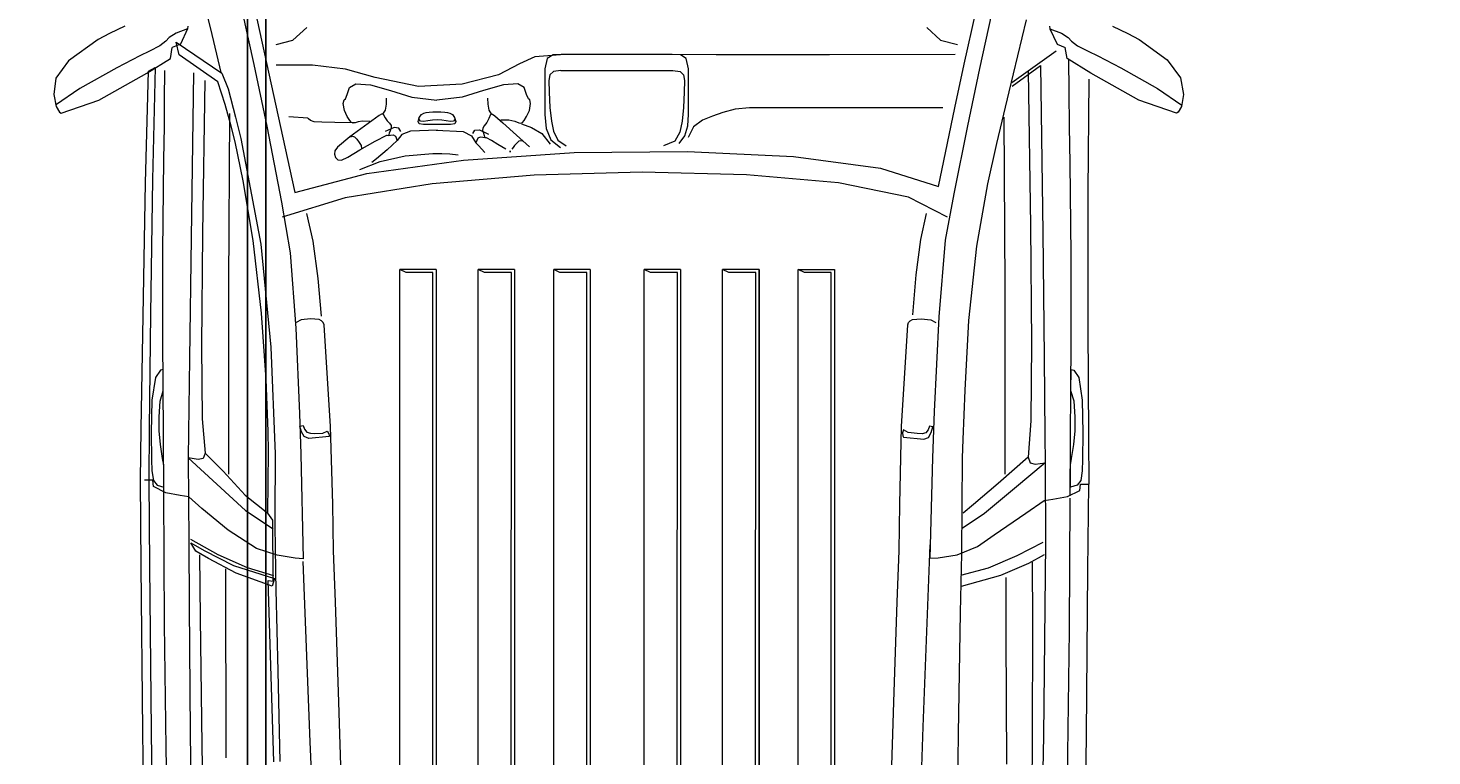
# Model space of a CAD drawing. Units: inches. Extents: x -10 to 502, y -868 to 56.
# Tile 4 of 14: x 78 to 165, y -671 to -626. Entities that reach past the tile are written whole.
import ezdxf

# ---------------------------------------------------------------- set-up
doc = ezdxf.new("R2010")
doc.units = ezdxf.units.IN
doc.header["$MEASUREMENT"] = 0
doc.layers.add('A-ANNO-DIMS', color=2, linetype='Continuous', lineweight=18)
doc.layers.add('C-PRKG-VEHI', color=8, linetype='Continuous', lineweight=13)
doc.styles.get("Standard").update_dxf_attribs({"font": 'arial.ttf'})
doc.dimstyles.get("Standard").update_dxf_attribs({"dimtxt": 0.18, "dimasz": 0.18, "dimexe": 0.18, "dimexo": 0.0625, "dimgap": 0.09, "dimtad": 0, "dimtih": 1, "dimtoh": 1, "dimdec": 0, "dimzin": 0, "dimdsep": 46, "dimlunit": 3, "dimtxsty": 'Standard', "dimcen": 0.09, "dimadec": 0, "dimazin": 0, "dimtfac": 1, "dimtdec": 0, "dimtofl": 0, "dimtmove": 0, "dimatfit": 3, "dimfxl": 1, "dimtolj": 1, "dimtzin": 0, "dimarcsym": 0})

# ---------------------------------------------------------------- blocks, each defined once
blk = doc.blocks.new('*D47')
at = {"layer": 'A-ANNO-DIMS', "color": 0, "lineweight": -2, "transparency": 16777216}
for p, q in [((91.951, -494.915), (91.951, -846.583)), ((201.951, -494.915), (201.951, -846.583)), ((92.131, -846.403), (146.622, -846.403)), ((201.771, -846.403), (147.28, -846.403))]:
    blk.add_line(p, q, dxfattribs=at)
at = {"layer": 'A-ANNO-DIMS', "color": 0, "transparency": 16777216}
for points in [[(92.131, -846.373), (92.131, -846.433), (91.951, -846.403)], [(201.771, -846.373), (201.771, -846.433), (201.951, -846.403)]]:
    blk.add_solid(points, dxfattribs=at)
at = {"layer": 'Defpoints', "color": 0, "transparency": 16777216}
for p in [(91.951, -494.853), (201.951, -494.853), (201.951, -846.403)]:
    blk.add_point(p, dxfattribs=at)
at = {"layer": 'A-ANNO-DIMS', "color": 0, "transparency": 16777216, "insert": (146.951, -846.403), "char_height": 0.18, "attachment_point": 5}
blk.add_mtext('\\A1;9\'-2"', dxfattribs=at)
blk = doc.blocks.new('*D56')
at = {"layer": 'A-ANNO-DIMS', "color": 0, "lineweight": -2, "transparency": 16777216}
for p, q in [((43.951, -549.915), (43.951, -846.583)), ((93.073, -549.915), (93.073, -846.583)), ((44.131, -846.403), (68.179, -846.403)), ((92.893, -846.403), (68.845, -846.403))]:
    blk.add_line(p, q, dxfattribs=at)
at = {"layer": 'A-ANNO-DIMS', "color": 0, "transparency": 16777216}
for points in [[(44.131, -846.373), (44.131, -846.433), (43.951, -846.403)], [(92.893, -846.373), (92.893, -846.433), (93.073, -846.403)]]:
    blk.add_solid(points, dxfattribs=at)
at = {"layer": 'Defpoints', "color": 0, "transparency": 16777216}
for p in [(43.951, -549.853), (93.073, -549.853), (43.951, -846.403)]:
    blk.add_point(p, dxfattribs=at)
at = {"layer": 'A-ANNO-DIMS', "color": 0, "transparency": 16777216, "insert": (68.512, -846.403), "char_height": 0.18, "attachment_point": 5}
blk.add_mtext('\\A1;4\'-1"', dxfattribs=at)

msp = doc.modelspace()

# ---------------------------------------------------------------- linework, layer by layer
at = {"layer": 'C-PRKG-VEHI'}
for p, q in [((91.361, -620.053), (94.882, -636.132)), ((89.054, -623.65), (89.645, -626.004)), ((91.587, -624.834), (92.343, -628.21)), ((136.301, -628.19), (137.028, -624.963)), ((138.01, -625.073), (137.254, -628.449)), ((140.152, -625.432), (139.073, -629.901)), ((83.408, -626.292), (82.704, -626.66)), ((84.355, -625.827), (83.408, -626.292)), ((87.097, -626.531), (86.898, -626.772)), ((87.52, -626.266), (87.097, -626.531)), ((88.24, -625.989), (87.52, -626.266)), ((88.24, -625.989), (87.793, -626.939)), ((88.255, -625.827), (88.24, -625.989)), ((89.645, -626.004), (90.296, -628.703)), ((94.753, -626.702), (95.608, -625.916)), ((133.998, -625.916), (134.853, -626.702)), ((141.602, -625.827), (141.616, -625.989)), ((141.616, -625.989), (142.064, -626.939)), ((141.616, -625.989), (142.337, -626.266)), ((142.337, -626.266), (142.759, -626.531)), ((142.759, -626.531), (142.958, -626.772)), ((145.502, -625.826), (146.449, -626.291)), ((146.449, -626.291), (147.152, -626.66)), ((82.704, -626.66), (80.86, -627.988)), ((85.871, -627.385), (85.276, -627.666)), ((86.527, -627.053), (85.871, -627.385)), ((86.898, -626.772), (86.527, -627.053)), ((87.178, -627.834), (87.29, -627.163)), ((87.793, -626.939), (87.29, -627.163)), ((87.524, -626.83), (90.362, -628.736)), ((87.719, -627.61), (87.524, -626.83)), ((93.719, -626.973), (94.753, -626.702)), ((134.853, -626.702), (135.888, -626.973)), ((142.008, -627.387), (139.267, -629.344)), ((142.064, -626.939), (142.567, -627.163)), ((142.679, -627.834), (142.567, -627.163)), ((142.958, -626.772), (143.329, -627.053)), ((143.329, -627.053), (143.986, -627.385)), ((143.986, -627.385), (144.58, -627.666)), ((147.152, -626.66), (148.869, -627.925)), ((80.86, -627.988), (80.085, -629.062)), ((85.276, -627.666), (83.852, -628.409)), ((85.708, -628.751), (87.178, -627.834)), ((90.102, -629.278), (87.719, -627.61)), ((92.343, -628.21), (93.133, -632.028)), ((95.965, -628.238), (93.721, -628.238)), ((98.01, -628.498), (95.965, -628.238)), ((108.782, -628.175), (107.474, -628.845)), ((109.731, -627.728), (108.782, -628.175)), ((111.589, -627.577), (109.731, -627.728)), ((110.499, -627.831), (110.359, -628.471)), ((110.862, -627.606), (110.499, -627.831)), ((111.366, -627.58), (110.862, -627.606)), ((118.241, -627.58), (111.366, -627.58)), ((115.309, -627.597), (111.589, -627.577)), ((120.959, -627.608), (115.309, -627.597)), ((118.744, -627.606), (118.241, -627.58)), ((119.108, -627.831), (118.744, -627.606)), ((119.247, -628.471), (119.108, -627.831)), ((127.966, -627.607), (120.959, -627.608)), ((135.754, -627.588), (127.966, -627.607)), ((135.731, -630.893), (136.301, -628.19)), ((139.278, -629.537), (141.031, -628.269)), ((141.031, -628.269), (141.171, -638.598)), ((144.149, -628.751), (142.679, -627.834)), ((142.77, -627.863), (142.793, -629.899)), ((144.58, -627.666), (146.005, -628.409)), ((148.869, -627.925), (149.708, -629.031)), ((80.085, -629.062), (79.958, -630.053)), ((83.852, -628.409), (81.568, -629.683)), ((82.732, -630.422), (85.708, -628.751)), ((85.634, -635.538), (85.813, -628.628)), ((85.813, -628.628), (86.224, -628.382)), ((86.224, -628.382), (86.062, -635.328)), ((86.806, -628.579), (86.788, -630.372)), ((88.604, -628.72), (88.46, -638.93)), ((89.297, -629.195), (89.16, -638.641)), ((90.362, -628.736), (90.741, -629.702)), ((99.849, -629.018), (98.01, -628.498)), ((102.536, -629.558), (99.849, -629.018)), ((107.474, -628.845), (105.231, -629.428)), ((110.359, -628.471), (110.359, -631.29)), ((110.663, -628.84), (110.604, -629.205)), ((110.885, -628.644), (110.663, -628.84)), ((111.337, -628.586), (110.885, -628.644)), ((111.337, -628.586), (118.269, -628.586)), ((118.269, -628.586), (118.722, -628.644)), ((118.722, -628.644), (118.944, -628.84)), ((118.944, -628.84), (119.003, -629.205)), ((119.247, -631.29), (119.247, -628.471)), ((137.254, -628.449), (136.512, -632.004)), ((140.274, -628.617), (140.416, -638.191)), ((144.036, -629.104), (143.959, -636.092)), ((147.124, -630.422), (144.149, -628.751)), ((146.005, -628.409), (148.288, -629.683)), ((149.708, -629.031), (149.899, -630.053)), ((79.958, -630.053), (80.098, -630.805)), ((81.568, -629.683), (80.069, -630.724)), ((90.559, -630.675), (90.102, -629.278)), ((90.741, -629.702), (91.21, -631.459)), ((98.011, -630.34), (98.119, -630.067)), ((98.119, -630.067), (98.265, -629.63)), ((98.265, -629.63), (98.654, -629.403)), ((98.654, -629.403), (99.558, -629.463)), ((99.558, -629.463), (100.797, -629.812)), ((100.797, -629.812), (102.116, -630.218)), ((105.231, -629.428), (102.536, -629.558)), ((106.545, -629.812), (105.227, -630.218)), ((107.784, -629.463), (106.545, -629.812)), ((108.688, -629.403), (107.784, -629.463)), ((109.077, -629.63), (108.688, -629.403)), ((109.223, -630.067), (109.077, -629.63)), ((109.331, -630.34), (109.223, -630.067)), ((110.604, -629.205), (110.619, -629.915)), ((110.619, -629.915), (110.67, -630.877)), ((118.987, -629.915), (118.937, -630.877)), ((119.003, -629.205), (118.987, -629.915)), ((139.073, -629.901), (138.317, -633.091)), ((142.793, -629.899), (142.81, -632.052)), ((148.288, -629.683), (149.787, -630.724)), ((149.899, -630.053), (149.758, -630.805)), ((80.098, -630.805), (80.301, -631.146)), ((80.405, -631.227), (82.732, -630.422)), ((86.788, -630.372), (86.782, -632.047)), ((90.941, -632.025), (90.559, -630.675)), ((97.875, -630.614), (97.926, -630.389)), ((97.941, -631.046), (97.875, -630.614)), ((97.926, -630.389), (98.011, -630.34)), ((100.52, -630.671), (100.46, -631.041)), ((100.536, -630.283), (100.52, -630.671)), ((102.116, -630.218), (103.671, -630.413)), ((105.227, -630.218), (103.671, -630.413)), ((106.806, -630.283), (106.825, -630.669)), ((106.825, -630.669), (106.889, -631.039)), ((109.417, -630.389), (109.331, -630.34)), ((109.401, -631.046), (109.467, -630.614)), ((109.467, -630.614), (109.417, -630.389)), ((110.67, -630.877), (110.762, -631.721)), ((118.937, -630.877), (118.845, -631.721)), ((123.026, -630.881), (122.132, -630.967)), ((134.982, -630.881), (123.026, -630.881)), ((135.053, -634.161), (135.731, -630.893)), ((149.452, -631.227), (147.124, -630.422)), ((149.758, -630.805), (149.555, -631.146)), ((80.301, -631.146), (80.405, -631.227)), ((90.833, -631.23), (90.768, -641.791)), ((91.21, -631.459), (91.533, -632.791)), ((95.69, -631.531), (94.501, -631.444)), ((95.724, -631.577), (95.69, -631.531)), ((95.844, -631.672), (95.724, -631.577)), ((96.08, -631.747), (95.844, -631.672)), ((96.54, -631.782), (96.08, -631.747)), ((97.359, -631.802), (96.54, -631.782)), ((98.608, -631.808), (97.359, -631.802)), ((98.116, -631.414), (97.941, -631.046)), ((98.278, -631.664), (98.116, -631.414)), ((98.383, -631.791), (98.278, -631.664)), ((98.484, -631.834), (98.383, -631.791)), ((98.608, -631.808), (98.484, -631.834)), ((98.786, -631.751), (98.608, -631.808)), ((99.069, -631.716), (98.786, -631.751)), ((99.515, -631.736), (99.069, -631.716)), ((100.09, -631.362), (99.41, -631.863)), ((100.23, -631.27), (100.09, -631.362)), ((100.286, -631.27), (100.23, -631.27)), ((100.296, -631.286), (100.286, -631.27)), ((100.46, -631.041), (100.296, -631.286)), ((100.353, -631.289), (100.457, -631.509)), ((100.457, -631.509), (100.598, -631.686)), ((100.598, -631.686), (100.743, -631.841)), ((102.501, -631.725), (102.578, -631.491)), ((102.569, -631.872), (102.501, -631.725)), ((102.569, -631.609), (102.578, -631.491)), ((102.655, -631.714), (102.569, -631.609)), ((102.578, -631.491), (102.716, -631.294)), ((102.837, -631.736), (102.655, -631.714)), ((102.716, -631.294), (102.863, -631.209)), ((103.099, -631.691), (102.837, -631.736)), ((102.863, -631.209), (103.01, -631.175)), ((103.01, -631.175), (103.191, -631.151)), ((103.395, -631.652), (103.099, -631.691)), ((103.191, -631.151), (103.423, -631.137)), ((103.686, -631.635), (103.395, -631.652)), ((103.423, -631.137), (103.671, -631.132)), ((103.671, -631.132), (103.919, -631.137)), ((103.968, -631.652), (103.686, -631.635)), ((103.919, -631.137), (104.152, -631.151)), ((104.251, -631.691), (103.968, -631.652)), ((104.152, -631.151), (104.333, -631.175)), ((104.505, -631.736), (104.251, -631.691)), ((104.333, -631.175), (104.48, -631.209)), ((104.48, -631.209), (104.627, -631.294)), ((104.688, -631.714), (104.505, -631.736)), ((104.627, -631.294), (104.764, -631.491)), ((104.774, -631.609), (104.688, -631.714)), ((104.764, -631.491), (104.841, -631.725)), ((104.764, -631.491), (104.774, -631.609)), ((104.841, -631.725), (104.774, -631.872)), ((106.751, -631.803), (106.605, -631.995)), ((106.886, -631.549), (106.751, -631.803)), ((106.993, -631.29), (106.886, -631.549)), ((106.889, -631.039), (107.051, -631.29)), ((107.051, -631.29), (107.062, -631.274)), ((107.062, -631.274), (107.117, -631.277)), ((107.117, -631.277), (107.252, -631.376)), ((107.252, -631.376), (107.744, -631.815)), ((107.626, -631.621), (108.124, -631.631)), ((108.124, -631.631), (108.504, -631.721)), ((108.504, -631.721), (108.734, -631.808)), ((108.734, -631.808), (108.858, -631.834)), ((108.858, -631.834), (108.96, -631.791)), ((108.96, -631.791), (109.064, -631.664)), ((109.064, -631.664), (109.226, -631.414)), ((109.226, -631.414), (109.401, -631.046)), ((110.359, -631.29), (110.434, -632.161)), ((110.762, -631.721), (110.89, -632.327)), ((118.845, -631.721), (118.709, -632.385)), ((119.199, -632.011), (119.247, -631.29)), ((120.121, -631.661), (119.555, -632.071)), ((120.73, -631.4), (120.121, -631.661)), ((121.364, -631.169), (120.73, -631.4)), ((122.132, -630.967), (121.364, -631.169)), ((138.764, -631.469), (138.828, -641.968)), ((149.555, -631.146), (149.452, -631.227)), ((86.782, -632.047), (86.751, -634.082)), ((91.185, -632.982), (90.941, -632.025)), ((93.133, -632.028), (94.05, -636.718)), ((99.41, -631.863), (98.289, -632.689)), ((98.337, -632.68), (98.449, -632.649)), ((98.449, -632.649), (98.564, -632.686)), ((99.844, -632.956), (100.575, -632.581)), ((101.029, -632.101), (100.458, -632.345)), ((100.575, -632.581), (100.596, -632.588)), ((100.596, -632.588), (100.664, -632.595)), ((100.664, -632.595), (100.791, -632.578)), ((100.692, -632.544), (100.691, -632.573)), ((100.712, -632.455), (100.692, -632.544)), ((100.777, -632.304), (100.712, -632.455)), ((100.743, -631.841), (100.834, -631.988)), ((100.841, -632.137), (100.777, -632.304)), ((100.791, -632.578), (100.959, -632.56)), ((100.834, -631.988), (100.841, -632.137)), ((100.959, -632.56), (101.111, -632.641)), ((101.322, -632.14), (101.029, -632.101)), ((101.111, -632.641), (101.205, -632.917)), ((101.506, -632.536), (101.205, -632.917)), ((101.437, -632.353), (101.322, -632.14)), ((102.041, -632.33), (101.506, -632.536)), ((103.714, -632.268), (102.041, -632.33)), ((102.837, -631.923), (102.569, -631.872)), ((104.505, -631.923), (102.837, -631.923)), ((103.628, -632.268), (105.295, -632.358)), ((104.774, -631.872), (104.505, -631.923)), ((105.295, -632.358), (105.811, -632.62)), ((105.811, -632.62), (106.087, -633.045)), ((105.886, -632.469), (106.012, -632.263)), ((106.012, -632.263), (106.307, -632.239)), ((106.307, -632.239), (106.864, -632.512)), ((106.507, -632.136), (106.492, -632.285)), ((106.492, -632.285), (106.548, -632.455)), ((106.605, -631.995), (106.507, -632.136)), ((106.548, -632.455), (106.605, -632.609)), ((106.605, -632.609), (106.62, -632.699)), ((107.744, -631.815), (108.604, -632.583)), ((108.604, -632.583), (109.393, -633.309)), ((108.903, -631.877), (109.527, -632.106)), ((109.527, -632.106), (110.171, -632.471)), ((110.171, -632.471), (110.679, -633.133)), ((110.434, -632.161), (110.722, -632.867)), ((110.89, -632.327), (111.155, -632.88)), ((118.709, -632.385), (118.394, -632.944)), ((118.66, -633.103), (119.02, -632.63)), ((119.02, -632.63), (119.199, -632.011)), ((119.555, -632.071), (119.235, -632.722)), ((136.512, -632.004), (135.673, -636.205)), ((142.81, -632.052), (142.846, -634.321)), ((91.686, -635.402), (91.185, -632.982)), ((91.533, -632.791), (92.765, -639.325)), ((97.359, -633.541), (97.327, -633.76)), ((97.512, -633.314), (97.359, -633.541)), ((98.289, -632.689), (97.512, -633.314)), ((98.156, -633.938), (98.891, -633.486)), ((98.564, -632.686), (98.704, -632.829)), ((98.704, -632.829), (98.863, -633.034)), ((98.863, -633.034), (98.98, -633.228)), ((98.891, -633.486), (99.844, -632.956)), ((98.98, -633.228), (99.005, -633.406)), ((100.585, -633.483), (99.941, -634.034)), ((101.205, -632.917), (100.585, -633.483)), ((106.196, -632.774), (106.087, -633.045)), ((106.087, -633.045), (106.256, -633.23)), ((106.353, -632.702), (106.196, -632.774)), ((106.256, -633.23), (106.429, -633.42)), ((106.519, -632.728), (106.353, -632.702)), ((106.429, -633.42), (106.635, -633.644)), ((106.645, -632.751), (106.519, -632.728)), ((106.62, -632.699), (106.619, -632.728)), ((106.714, -632.748), (106.645, -632.751)), ((106.734, -632.742), (106.714, -632.748)), ((107.042, -632.914), (106.734, -632.742)), ((107.451, -633.156), (107.042, -632.914)), ((107.93, -633.452), (107.451, -633.156)), ((108.383, -633.333), (108.305, -633.45)), ((108.482, -633.212), (108.383, -633.333)), ((108.59, -633.088), (108.482, -633.212)), ((108.738, -632.952), (108.59, -633.088)), ((108.854, -632.922), (108.738, -632.952)), ((108.964, -632.958), (108.854, -632.922)), ((110.722, -632.867), (111.317, -633.335)), ((111.155, -632.88), (111.679, -633.245)), ((118.394, -632.944), (117.693, -633.234)), ((138.317, -633.091), (137.755, -635.597)), ((86.751, -634.082), (86.686, -639.751)), ((97.327, -633.76), (97.392, -633.956)), ((97.392, -633.956), (97.531, -634.105)), ((97.531, -634.105), (97.769, -634.131)), ((97.769, -634.131), (98.156, -633.938)), ((98.899, -634.705), (100.153, -634.206)), ((99.341, -634.943), (105.324, -634.117)), ((99.941, -634.034), (99.644, -634.281)), ((100.153, -634.206), (101.703, -633.854)), ((101.703, -633.854), (103.427, -633.72)), ((103.427, -633.72), (103.983, -633.722)), ((103.983, -633.722), (104.476, -633.743)), ((104.476, -633.743), (104.993, -633.802)), ((105.324, -634.117), (112.164, -633.662)), ((108.159, -633.588), (108.24, -633.582)), ((108.186, -633.586), (108.159, -633.588)), ((108.213, -633.584), (108.186, -633.586)), ((108.24, -633.582), (108.213, -633.584)), ((112.164, -633.662), (119.192, -633.589)), ((119.192, -633.589), (125.741, -633.906)), ((125.741, -633.906), (131.141, -634.623)), ((134.725, -635.749), (135.053, -634.161)), ((142.846, -634.321), (142.911, -639.99)), ((94.882, -636.132), (99.341, -634.943)), ((109.697, -635.064), (103.378, -635.598)), ((116.374, -634.87), (109.697, -635.064)), ((122.84, -635.025), (116.374, -634.87)), ((128.526, -635.535), (122.84, -635.025)), ((131.141, -634.623), (134.725, -635.749)), ((85.476, -643.767), (85.634, -635.538)), ((86.062, -635.328), (85.941, -643.642)), ((92.287, -639.103), (91.686, -635.402)), ((103.378, -635.598), (97.988, -636.465)), ((132.861, -636.409), (128.526, -635.535)), ((137.755, -635.597), (137.07, -639.458)), ((143.959, -636.092), (143.962, -644.369)), ((94.05, -636.718), (94.596, -639.857)), ((97.988, -636.465), (94.095, -637.655)), ((135.277, -637.655), (132.861, -636.409)), ((135.673, -636.205), (135.144, -639.077)), ((95.604, -637.422), (95.984, -639.141)), ((133.952, -637.422), (133.602, -639.032)), ((89.16, -638.641), (89.1, -645.612)), ((140.416, -638.191), (140.484, -645.443)), ((141.171, -638.598), (141.259, -646.326)), ((88.46, -638.93), (88.359, -646.397)), ((92.809, -643.596), (92.287, -639.103)), ((92.765, -639.325), (93.384, -645.691)), ((95.984, -639.141), (96.306, -641.451)), ((133.602, -639.032), (133.326, -641.214)), ((135.144, -639.077), (134.746, -643.814)), ((137.07, -639.458), (136.583, -644.052)), ((86.686, -639.751), (86.684, -645.358)), ((94.596, -639.857), (94.944, -644.513)), ((142.911, -639.99), (142.913, -645.597)), ((101.758, -641.088), (101.376, -640.902)), ((103.631, -640.902), (101.376, -640.902)), ((101.378, -699.991), (101.378, -640.902)), ((103.426, -641.088), (101.758, -641.088)), ((103.405, -699.052), (103.426, -641.088)), ((103.629, -640.902), (103.629, -699.991)), ((103.631, -640.902), (103.631, -699.991)), ((106.611, -641.088), (106.228, -640.902)), ((108.483, -640.902), (106.228, -640.902)), ((106.23, -699.991), (106.23, -640.902)), ((108.278, -641.088), (106.611, -641.088)), ((108.257, -699.052), (108.278, -641.088)), ((108.481, -640.902), (108.481, -699.991)), ((108.483, -640.902), (108.483, -699.991)), ((111.289, -641.088), (110.907, -640.902)), ((113.161, -640.902), (110.907, -640.902)), ((110.909, -699.991), (110.909, -640.902)), ((112.957, -641.088), (111.289, -641.088)), ((112.935, -699.052), (112.957, -641.088)), ((113.159, -640.902), (113.159, -699.991)), ((113.161, -640.902), (113.161, -699.991)), ((116.887, -641.088), (116.504, -640.902)), ((118.759, -640.902), (116.504, -640.902)), ((116.506, -699.991), (116.506, -640.902)), ((118.555, -641.088), (116.887, -641.088)), ((118.533, -699.052), (118.555, -641.088)), ((118.757, -640.902), (118.757, -699.991)), ((118.759, -640.902), (118.759, -699.991)), ((121.739, -641.088), (121.356, -640.902)), ((123.611, -640.902), (121.356, -640.902)), ((121.358, -699.991), (121.358, -640.902)), ((123.407, -641.088), (121.739, -641.088)), ((123.385, -699.052), (123.407, -641.088)), ((123.609, -640.902), (123.609, -699.991)), ((123.611, -640.902), (123.611, -699.991)), ((126.037, -699.991), (126.037, -640.902)), ((126.419, -641.088), (126.037, -640.902)), ((126.037, -640.902), (128.29, -640.902)), ((128.087, -641.088), (126.419, -641.088)), ((128.065, -699.052), (128.087, -641.088)), ((128.29, -640.902), (128.29, -699.991)), ((133.326, -641.214), (133.12, -643.704)), ((90.768, -641.791), (90.764, -650.156)), ((96.306, -641.451), (96.513, -643.79)), ((138.828, -641.968), (138.83, -650.218)), ((85.362, -650.751), (85.476, -643.767)), ((85.941, -643.642), (85.865, -650.711)), ((93.091, -647.709), (92.809, -643.596)), ((95.855, -643.942), (95.262, -644.007)), ((96.39, -643.994), (95.855, -643.942)), ((133.113, -643.994), (133.648, -643.942)), ((133.648, -643.942), (134.241, -644.007)), ((134.746, -643.814), (134.457, -649.681)), ((94.944, -644.513), (95.17, -649.797)), ((95.262, -644.007), (94.952, -644.181)), ((96.527, -644.062), (96.39, -643.994)), ((96.637, -644.174), (96.527, -644.062)), ((96.687, -644.31), (96.637, -644.174)), ((97.092, -650.609), (96.687, -644.31)), ((132.425, -650.609), (132.816, -644.31)), ((132.816, -644.31), (132.866, -644.174)), ((132.866, -644.174), (132.976, -644.062)), ((132.976, -644.062), (133.113, -643.994)), ((134.241, -644.007), (134.551, -644.181)), ((136.583, -644.052), (136.357, -648.368)), ((143.962, -644.369), (143.998, -651.281)), ((86.684, -645.358), (86.695, -647.895)), ((89.1, -645.612), (89.146, -650.14)), ((93.384, -645.691), (93.665, -652.308)), ((140.484, -645.443), (140.447, -650.252)), ((142.913, -645.597), (142.902, -648.135)), ((88.359, -646.397), (88.301, -650.982)), ((141.259, -646.326), (141.306, -651.171)), ((86.558, -647.116), (86.245, -647.568)), ((86.717, -647.084), (86.558, -647.116)), ((86.73, -648.403), (86.717, -647.084)), ((142.922, -648.403), (142.935, -647.084)), ((142.935, -647.084), (143.093, -647.116)), ((143.093, -647.116), (143.406, -647.568)), ((86.245, -647.568), (86.026, -648.975)), ((86.695, -647.895), (86.751, -654.662)), ((93.215, -650.894), (93.091, -647.709)), ((142.902, -648.135), (142.846, -654.901)), ((143.406, -647.568), (143.625, -648.975)), ((86.026, -648.975), (85.988, -650.996)), ((86.476, -650.006), (86.53, -649.05)), ((86.53, -649.05), (86.73, -648.403)), ((136.357, -648.368), (136.231, -651.405)), ((143.121, -649.05), (142.922, -648.403)), ((143.175, -650.006), (143.121, -649.05)), ((143.625, -648.975), (143.663, -650.996)), ((86.478, -650.867), (86.476, -650.006)), ((95.17, -649.797), (95.251, -652.313)), ((134.457, -649.681), (134.346, -652.553)), ((143.173, -650.867), (143.175, -650.006)), ((85.316, -653.922), (85.362, -650.751)), ((85.865, -650.711), (85.836, -653.922)), ((86.551, -651.718), (86.478, -650.867)), ((89.146, -650.14), (89.323, -652.257)), ((90.764, -650.156), (90.773, -653.559)), ((93.243, -652.173), (93.215, -650.894)), ((95.192, -650.578), (95.386, -650.538)), ((95.282, -650.934), (95.192, -650.578)), ((95.386, -650.538), (95.467, -650.767)), ((95.467, -650.767), (95.622, -650.959)), ((96.612, -651.022), (96.873, -650.907)), ((96.873, -650.907), (96.971, -651.053)), ((97.218, -655.407), (97.092, -650.609)), ((132.324, -655.407), (132.425, -650.609)), ((132.553, -650.821), (132.489, -651)), ((132.847, -650.97), (132.553, -650.821)), ((134.089, -650.811), (133.933, -651.002)), ((134.171, -650.581), (134.089, -650.811)), ((134.364, -650.621), (134.171, -650.581)), ((134.274, -650.977), (134.364, -650.621)), ((138.83, -650.218), (138.82, -653.559)), ((140.447, -650.252), (140.274, -652.496)), ((143.1, -651.718), (143.173, -650.867)), ((85.988, -650.996), (86.01, -652.656)), ((86.686, -652.587), (86.551, -651.718)), ((88.301, -650.982), (88.282, -652.541)), ((95.449, -651.236), (95.282, -650.934)), ((95.743, -651.341), (95.449, -651.236)), ((95.622, -650.959), (95.853, -651.021)), ((97, -651.218), (95.743, -651.341)), ((95.853, -651.021), (96.119, -651.034)), ((96.119, -651.034), (96.612, -651.022)), ((96.971, -651.053), (97, -651.17)), ((97, -651.17), (97, -651.218)), ((132.489, -651), (132.522, -651.179)), ((132.522, -651.179), (132.556, -651.261)), ((132.556, -651.261), (133.813, -651.385)), ((133.403, -651.044), (132.847, -650.97)), ((133.703, -651.065), (133.403, -651.044)), ((133.933, -651.002), (133.703, -651.065)), ((133.813, -651.385), (134.107, -651.279)), ((134.107, -651.279), (134.274, -650.977)), ((136.231, -651.405), (136.191, -652.553)), ((141.306, -651.171), (141.32, -652.848)), ((142.965, -652.587), (143.1, -651.718)), ((143.663, -650.996), (143.642, -652.656)), ((143.998, -651.281), (144.021, -654.174)), ((86.01, -652.656), (86.03, -653.345)), ((86.759, -652.985), (86.686, -652.587)), ((88.282, -652.541), (90.046, -654.173)), ((88.888, -652.654), (88.282, -652.541)), ((88.282, -652.541), (88.304, -657.74)), ((89.202, -652.592), (88.888, -652.654)), ((89.323, -652.257), (89.202, -652.592)), ((89.323, -652.257), (90.443, -653.379)), ((93.209, -655.98), (93.243, -652.173)), ((93.665, -652.308), (93.639, -656.197)), ((95.251, -652.313), (95.381, -658.807)), ((134.346, -652.553), (134.182, -658.762)), ((136.191, -652.553), (136.139, -658.482)), ((140.274, -652.496), (138.42, -654.128)), ((140.274, -652.496), (140.396, -652.849)), ((142.893, -652.985), (142.965, -652.587)), ((143.642, -652.656), (143.621, -653.345)), ((86.03, -653.345), (86.119, -653.951)), ((86.759, -654.357), (86.759, -652.985)), ((90.443, -653.379), (91.807, -654.849)), ((141.32, -652.848), (139.432, -654.45)), ((140.396, -652.849), (140.713, -652.944)), ((140.713, -652.944), (141.32, -652.848)), ((141.32, -652.848), (141.337, -657.807)), ((142.893, -654.357), (142.893, -652.985)), ((143.621, -653.345), (143.533, -653.951)), ((85.362, -659.257), (85.316, -653.922)), ((86.079, -653.935), (85.576, -653.922)), ((85.836, -653.922), (85.882, -659.252)), ((86.135, -654.327), (86.079, -653.935)), ((86.119, -653.951), (86.352, -654.249)), ((86.884, -654.716), (86.135, -654.327)), ((86.352, -654.249), (86.759, -654.357)), ((90.046, -654.173), (91.819, -655.813)), ((138.42, -654.128), (136.888, -655.433)), ((143.299, -654.249), (142.893, -654.357)), ((143.533, -653.951), (143.299, -654.249)), ((143.462, -654.566), (143.518, -654.174)), ((143.518, -654.174), (144.001, -654.174)), ((143.975, -659.503), (144.021, -654.174)), ((86.751, -654.662), (86.794, -662.836)), ((87.779, -654.875), (86.884, -654.716)), ((88.304, -654.967), (87.779, -654.875)), ((89.12, -655.681), (88.304, -654.967)), ((91.807, -654.849), (93.209, -655.98)), ((139.432, -654.45), (137.561, -655.986)), ((140.122, -655.973), (141.264, -655.184)), ((141.264, -655.184), (141.796, -655.098)), ((141.796, -655.098), (142.705, -654.949)), ((142.705, -654.949), (143.462, -654.566)), ((142.854, -655.053), (142.81, -663.227)), ((90.758, -657.027), (89.12, -655.681)), ((91.819, -655.813), (93.524, -656.938)), ((93.514, -656.41), (93.209, -655.98)), ((97.274, -658.302), (97.218, -655.407)), ((132.282, -658.302), (132.324, -655.407)), ((137.561, -655.986), (136.195, -656.917)), ((136.888, -655.433), (136.251, -655.966)), ((138.176, -657.321), (140.122, -655.973)), ((93.535, -660.187), (93.514, -656.41)), ((93.639, -656.197), (93.666, -658.672)), ((88.304, -657.74), (88.326, -661.677)), ((88.425, -657.581), (90.107, -658.524)), ((88.737, -658.325), (88.434, -657.805)), ((88.434, -657.805), (89.258, -658.281)), ((92.506, -658.151), (90.758, -657.027)), ((137.146, -658.035), (138.176, -657.321)), ((141.181, -657.79), (139.575, -658.611)), ((141.337, -657.807), (141.304, -661.788)), ((89.535, -658.781), (88.737, -658.325)), ((88.975, -658.541), (89.018, -662.47)), ((89.258, -658.281), (91.087, -659.214)), ((90.107, -658.524), (91.924, -659.324)), ((93.791, -658.572), (92.506, -658.151)), ((93.666, -658.672), (93.671, -658.924)), ((94.905, -658.762), (93.791, -658.572)), ((97.389, -661.46), (97.274, -658.302)), ((132.167, -661.46), (132.282, -658.302)), ((134.178, -657.921), (133.76, -669.192)), ((134.182, -658.762), (134.701, -658.739)), ((134.701, -658.739), (135.878, -658.554)), ((135.878, -658.554), (137.146, -658.035)), ((136.139, -658.482), (136.066, -662.129)), ((139.575, -658.611), (137.791, -659.37)), ((140.311, -659.066), (141.281, -658.536)), ((85.457, -669.432), (85.362, -659.257)), ((85.882, -659.252), (85.977, -669.417)), ((91.235, -659.681), (89.535, -658.781)), ((90.578, -659.407), (90.594, -671.12)), ((91.087, -659.214), (93.622, -660.025)), ((91.924, -659.324), (93.546, -659.819)), ((93.671, -658.924), (93.685, -659.632)), ((95.381, -658.807), (94.905, -658.762)), ((95.364, -658.955), (95.805, -670.125)), ((137.791, -659.37), (136.083, -659.824)), ((138.586, -659.812), (140.311, -659.066)), ((140.527, -658.996), (140.535, -662.692)), ((143.88, -669.667), (143.975, -659.503)), ((93.471, -660.489), (91.235, -659.681)), ((93.385, -665.39), (93.221, -660.144)), ((93.221, -660.144), (93.535, -660.187)), ((93.622, -660.025), (93.471, -660.489)), ((93.685, -659.632), (93.705, -660.725)), ((136.139, -660.496), (138.586, -659.812)), ((138.881, -659.949), (138.898, -663.527)), ((93.705, -660.725), (93.816, -665.754)), ((88.326, -661.677), (88.388, -669.553)), ((97.591, -667.668), (97.389, -661.46)), ((131.965, -667.668), (132.167, -661.46)), ((136.066, -662.129), (135.93, -669.616)), ((141.304, -661.788), (141.221, -669.747)), ((86.794, -662.836), (86.89, -670.481)), ((89.018, -662.47), (89.118, -670.332)), ((140.535, -662.692), (140.529, -670.12)), ((138.898, -663.527), (138.935, -671.511)), ((142.81, -663.227), (142.714, -670.872)), ((93.57, -671.36), (93.385, -665.39)), ((93.816, -665.754), (93.941, -671.332)), ((97.837, -675.397), (97.591, -667.668)), ((131.719, -675.397), (131.965, -667.668)), ((85.54, -675.7), (85.457, -669.432)), ((85.977, -669.417), (86.06, -675.679)), ((88.388, -669.553), (88.484, -675.465)), ((133.76, -669.192), (133.495, -676.811)), ((135.93, -669.616), (135.856, -675.761)), ((141.221, -669.747), (141.113, -675.705)), ((143.797, -675.928), (143.88, -669.667)), ((86.89, -670.481), (86.986, -676.312)), ((89.118, -670.332), (89.235, -676.238)), ((95.805, -670.125), (96.096, -677.158)), ((140.529, -670.12), (140.463, -675.791)), ((142.714, -670.872), (142.618, -676.703))]:
    msp.add_line(p, q, dxfattribs=at)

# ---------------------------------------------------------------- dimensions: what is measured, and where the dimension line sits
at = {"layer": 'A-ANNO-DIMS'}
for base, p1, p2, picture, middle in [((201.951, -846.403), (91.951, -494.853), (201.951, -494.853), '*D47', (146.951, -846.403)), ((43.951, -846.403), (93.073, -549.853), (43.951, -549.853), '*D56', (68.512, -846.403))]:
    dim = msp.add_linear_dim(base=base, p1=p1, p2=p2, dimstyle='Standard', override={"dimdec": 1, "dimlfac": 1, "dimrnd": 0, "dimzin": 1, "dimdsep": 46, "dimlunit": 4, "dimfrac": 2}, dxfattribs=at)
    dim.commit()
    dim.dimension.update_dxf_attribs({"geometry": picture, "text_midpoint": middle})

doc.saveas('drawing.dxf')
